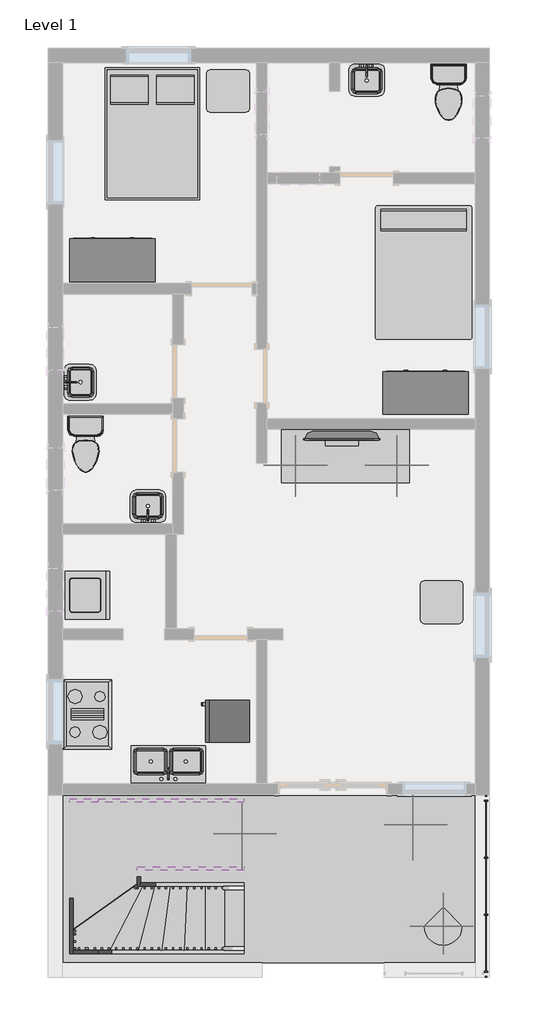
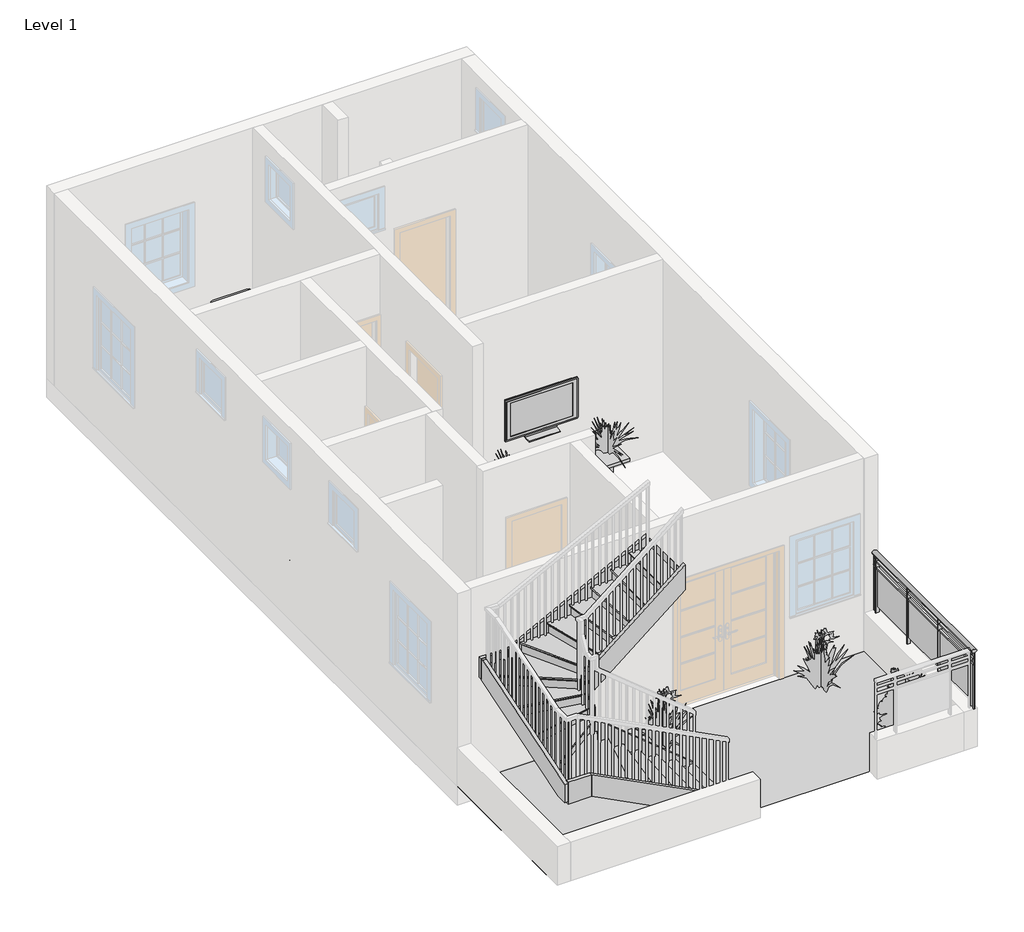
# One storey, part 3 of 3: 8 flow terminals, 8 furniture elements, 8 members, 5 geographic elements, 4 proxies, 1 railing, 1 stair flight.
"""IFC4 building model written with IfcOpenShell, lengths in millimetres."""

from ifc_helpers import new_model, si_unit, point, frame, origin, place, context, project, spatial, polyline, ellipse_curve, trimmed, outline, extrude, triangles, transform, mapped, element, save
from ifc_brep_helpers import plane_surface, extruded_surface, advanced_brep
from components import proxy_bb1e6e30, proxy_c523a7b7, proxy_718fa39f, flow_terminal_accce45a, flow_terminal_a53be723, flow_terminal_62a433f7, toilet_domestic_3d_toilet_domestic_3d_f7549cf7, toilet_domestic_3d_toilet_domestic_3d_183bbd19, furniture_c8abb964, furniture_0253826f, furniture_9fa109b2, furniture_7a3aaa4f, furniture_31d08a24, furniture_62ce4b1f, rpc_plant_tropical_55f6ff97, rpc_plant_tropical_agave_1_5_93a2a214, rpc_plant_tropical_jungle_flame_3_9c4808c2, stair_flight_52655b22

model = new_model("IFC4")

# Units and contexts
model_context = context("Model", 3, world=origin())
ifc_project = project(units=[si_unit("LENGTHUNIT", "METRE", prefix="MILLI")], contexts=[model_context])

# Site, building, storey
site = spatial("IfcSite", under=ifc_project)
building = spatial("IfcBuilding", under=site)
storey = spatial("IfcBuildingStorey", under=building, Name="Level 1", Elevation=0.0)

# Proxies
placement = place(None, origin())
element("IfcBuildingElementProxy", 1, Name="Building Element Proxy", at=placement, inside=storey, context=model_context, shape_type="Tessellation", body=[
    triangles([(-16060.3755066, 5665.9419479, 0.0), (-16060.3755066, 3354.5417542, 0.0), (-9761.1762817, 3354.5417542, 0.0), (-9761.1762817, 5665.9419479, 0.0), (-15857.1762817, 3278.3417542, 0.0), (-13012.3755066, 3278.3417542, 0.0), (-9964.3755066, 3278.3417542, 0.0)], [[1, 2, 5], [1, 5, 6], [6, 7, 4], [6, 4, 1], [3, 4, 7]], closed=False),
])
proxy_shape = proxy_bb1e6e30(model_context)
element("IfcBuildingElementProxy", 2, Name="Cook Top-4 Unit : 36\" x 20\"", ObjectType="Cook Top-4 Unit : 36\" x 20\"", at=placement, inside=storey, context=model_context, shape_type="MappedRepresentation", body=[
    mapped(proxy_shape, transform((-15501.5757671, 6821.6418963, 0.0), x_axis=(0.0, 1.0000000000000002, 0.0), y_axis=(-1.0000000000000002, 0.0, 0.0), z_axis=(0.0, 0.0, 1.0))),
])
proxy_2_shape = proxy_c523a7b7(model_context)
element("IfcBuildingElementProxy", 3, Name="Refrigerator : 24\" x 25\" LH", ObjectType="Refrigerator : 24\" x 25\" LH", at=placement, inside=storey, context=model_context, shape_type="MappedRepresentation", body=[
    mapped(proxy_2_shape, transform((-13488.6257671, 6725.1929248, 0.0), x_axis=(0.0, -1.0000000000000007, 0.0), y_axis=(1.0000000000000007, 0.0, 0.0), z_axis=(0.0, 0.0, 1.0))),
])
proxy_3_shape = proxy_718fa39f(model_context)
element("IfcBuildingElementProxy", 4, Name="Washer : 27\" x 25\" x 35\"", ObjectType="Washer : 27\" x 25\" x 35\"", at=placement, inside=storey, context=model_context, shape_type="MappedRepresentation", body=[
    mapped(proxy_3_shape, transform((-15782.2932356, 8942.7923315, 0.0), x_axis=(0.0, -1.0000000000000016, 0.0), y_axis=(1.0000000000000016, 0.0, 0.0), z_axis=(0.0, 0.0, 1.0))),
])

# Flow terminals
flow_terminal_shape = flow_terminal_accce45a(model_context)
element("IfcFlowTerminal", 5, ObjectType="Floor Drain - Round : 5\" Strainer - 2\" Drain", at=placement, inside=storey, context=model_context, shape_type="MappedRepresentation", body=[
    mapped(flow_terminal_shape, transform((-10294.5757671, 14873.4418963, 0.0), x_axis=(1.0, 0.0, 0.0), y_axis=(0.0, 1.0, 0.0), z_axis=(0.0, 0.0, 1.0))),
])
element("IfcFlowTerminal", 6, ObjectType="Floor Drain - Round : 5\" Strainer - 2\" Drain", at=placement, inside=storey, context=model_context, shape_type="MappedRepresentation", body=[
    mapped(flow_terminal_shape, transform((-15679.3757671, 12587.4418963, 0.0), x_axis=(1.0, 0.0, 0.0), y_axis=(0.0, 1.0, 0.0), z_axis=(0.0, 0.0, 1.0))),
])
flow_terminal_2_shape = flow_terminal_a53be723(model_context)
element("IfcFlowTerminal", 7, ObjectType="Sink Kitchen-Double : 42\" x 21\"", at=placement, inside=storey, context=model_context, shape_type="MappedRepresentation", body=[
    mapped(flow_terminal_2_shape, transform((-14330.1865265, 6112.7872974, 0.0), x_axis=(-1.0000000000000004, 0.0, 0.0), y_axis=(0.0, -1.0000000000000004, 0.0), z_axis=(0.0, 0.0, 1.0))),
])
flow_terminal_3_shape = flow_terminal_62a433f7(model_context)
element("IfcFlowTerminal", 8, ObjectType="Sink Vanity-Square : 20\" x 18\"", at=placement, inside=storey, context=model_context, shape_type="MappedRepresentation", body=[
    mapped(flow_terminal_3_shape, transform((-11529.4650076, 15912.4964952, 0.0), x_axis=(1.0, 0.0, 0.0), y_axis=(0.0, 1.0, 0.0), z_axis=(0.0, 0.0, 1.0))),
])
element("IfcFlowTerminal", 9, ObjectType="Sink Vanity-Square : 20\" x 18\"", at=placement, inside=storey, context=model_context, shape_type="MappedRepresentation", body=[
    mapped(flow_terminal_3_shape, transform((-15651.6303659, 11543.0526557, 0.0), x_axis=(0.0, 1.0, 0.0), y_axis=(-1.0, 0.0, 0.0), z_axis=(0.0, 0.0, 1.0))),
])
element("IfcFlowTerminal", 10, ObjectType="Sink Vanity-Square : 20\" x 18\"", at=placement, inside=storey, context=model_context, shape_type="MappedRepresentation", body=[
    mapped(flow_terminal_3_shape, transform((-14622.2865265, 9744.9872974, 0.0), x_axis=(-0.9999999999999998, 0.0, 0.0), y_axis=(0.0, -0.9999999999999998, 0.0), z_axis=(0.0, 0.0, 1.0))),
])
toilet_domestic_3d_toilet_domestic_3d_shape = toilet_domestic_3d_toilet_domestic_3d_f7549cf7(model_context)
toilet_domestic_3d_toilet_domestic_3d_2_shape = toilet_domestic_3d_toilet_domestic_3d_183bbd19(model_context)
element("IfcFlowTerminal", 11, ObjectType="Toilet-Domestic-3D : Toilet-Domestic-3D", at=placement, inside=storey, context=model_context, shape_type="MappedRepresentation", body=[
    mapped(toilet_domestic_3d_toilet_domestic_3d_shape, transform((-10345.3757671, 15597.9458689, 0.0), x_axis=(1.0, 0.0, 0.0), y_axis=(0.0, 1.0, 0.0), z_axis=(0.0, 0.0, 1.0))),
    mapped(toilet_domestic_3d_toilet_domestic_3d_2_shape, transform((-10345.3757671, 15597.9458689, 0.0), x_axis=(1.0, 0.0, 0.0), y_axis=(0.0, 1.0, 0.0), z_axis=(0.0, 0.0, 1.0))),
])
element("IfcFlowTerminal", 12, ObjectType="Toilet-Domestic-3D : Toilet-Domestic-3D", at=placement, inside=storey, context=model_context, shape_type="MappedRepresentation", body=[
    mapped(toilet_domestic_3d_toilet_domestic_3d_shape, transform((-15526.9757671, 10581.4458689, 0.0), x_axis=(1.0, 0.0, 0.0), y_axis=(0.0, 1.0, 0.0), z_axis=(0.0, 0.0, 1.0))),
    mapped(toilet_domestic_3d_toilet_domestic_3d_2_shape, transform((-15526.9757671, 10581.4458689, 0.0), x_axis=(1.0, 0.0, 0.0), y_axis=(0.0, 1.0, 0.0), z_axis=(0.0, 0.0, 1.0))),
])

# Furniture
furniture_shape = furniture_c8abb964(model_context)
element("IfcFurniture", 13, ObjectType="Bed-Box : Double 53\" x 74\"", at=placement, inside=storey, context=model_context, shape_type="MappedRepresentation", body=[
    mapped(furniture_shape, transform((-14913.6282261, 15336.4714045, 0.0), x_axis=(1.0, 0.0, 0.0), y_axis=(0.0, 1.0, 0.0), z_axis=(0.0, 0.0, 1.0))),
])
furniture_2_shape = furniture_0253826f(model_context)
element("IfcFurniture", 14, ObjectType="Bed-Standard.0001 : Double 54\" x 75\"", at=placement, inside=storey, context=model_context, shape_type="MappedRepresentation", body=[
    mapped(furniture_2_shape, transform((-10972.4642916, 13166.4369782, 0.0), x_axis=(1.0, 0.0, 0.0), y_axis=(0.0, 1.0, 0.0), z_axis=(0.0, 0.0, 1.0))),
])
furniture_3_shape = furniture_9fa109b2(model_context)
element("IfcFurniture", 15, ObjectType="Dresser : 48\" x 72\" x 24\"", at=placement, inside=storey, context=model_context, shape_type="MappedRepresentation", body=[
    mapped(furniture_3_shape, transform((-15415.1690269, 12935.4789422, 0.0), x_axis=(-1.0000000000000004, 0.0, 0.0), y_axis=(0.0, -1.0000000000000004, 0.0), z_axis=(0.0, 0.0, 1.0))),
])
element("IfcFurniture", 16, ObjectType="Dresser : 48\" x 72\" x 24\"", at=placement, inside=storey, context=model_context, shape_type="MappedRepresentation", body=[
    mapped(furniture_3_shape, transform((-10944.7690269, 11043.1789422, 0.0), x_axis=(-1.0000000000000004, 0.0, 0.0), y_axis=(0.0, -1.0000000000000004, 0.0), z_axis=(0.0, 0.0, 1.0))),
])
furniture_4_shape = furniture_7a3aaa4f(model_context)
element("IfcFurniture", 17, ObjectType="TV - Flat Screen : 42\"", at=placement, inside=storey, context=model_context, shape_type="MappedRepresentation", body=[
    mapped(furniture_4_shape, transform((-11865.4312529, 10801.7032726, 1041.4), x_axis=(1.0, 0.0, 0.0), y_axis=(0.0, 1.0, 0.0), z_axis=(0.0, 0.0, 1.0))),
])
furniture_5_shape = furniture_31d08a24(model_context)
element("IfcFurniture", 18, ObjectType="Table-End : 24\" x 24\"", at=placement, inside=storey, context=model_context, shape_type="MappedRepresentation", body=[
    mapped(furniture_5_shape, transform((-13803.5093973, 15559.2418963, 0.0), x_axis=(1.0, 0.0, 0.0), y_axis=(0.0, 1.0, 0.0), z_axis=(0.0, 0.0, 1.0))),
])
element("IfcFurniture", 19, ObjectType="Table-End : 24\" x 24\"", at=placement, inside=storey, context=model_context, shape_type="MappedRepresentation", body=[
    mapped(furniture_5_shape, transform((-10755.5093973, 8269.4418963, 0.0), x_axis=(1.0, 0.0, 0.0), y_axis=(0.0, 1.0, 0.0), z_axis=(0.0, 0.0, 1.0))),
])
furniture_6_shape = furniture_62ce4b1f(model_context)
element("IfcFurniture", 20, ObjectType="Table-Rectangular : 72\" x 30\"", at=placement, inside=storey, context=model_context, shape_type="MappedRepresentation", body=[
    mapped(furniture_6_shape, transform((-11818.5757671, 10504.6418963, 0.0), x_axis=(1.0, 0.0, 0.0), y_axis=(0.0, 1.0, 0.0), z_axis=(0.0, 0.0, 1.0))),
])

# Geographic elements
rpc_plant_tropical_shape = rpc_plant_tropical_55f6ff97(model_context)
element("IfcGeographicElement", 21, ObjectType="RPC Plant - Tropical", at=placement, inside=storey, context=model_context, shape_type="MappedRepresentation", body=[
    mapped(rpc_plant_tropical_shape, transform((-13291.7757671, 5119.8418963, 0.0), x_axis=(1.0, 0.0, 0.0), y_axis=(0.0, 1.0, 0.0), z_axis=(0.0, 0.0, 1.0))),
])
element("IfcGeographicElement", 22, ObjectType="RPC Plant - Tropical", at=placement, inside=storey, context=model_context, shape_type="MappedRepresentation", body=[
    mapped(rpc_plant_tropical_shape, transform((-10853.3757671, 5246.8418963, 0.0), x_axis=(1.0, 0.0, 0.0), y_axis=(0.0, 1.0, 0.0), z_axis=(0.0, 0.0, 1.0))),
])
rpc_plant_tropical_agave_1_5_shape = rpc_plant_tropical_agave_1_5_93a2a214(model_context)
element("IfcGeographicElement", 23, ObjectType="RPC Plant - Tropical : Agave - 1.5'", at=placement, inside=storey, context=model_context, shape_type="MappedRepresentation", body=[
    mapped(rpc_plant_tropical_agave_1_5_shape, transform((-12529.7757671, 10377.6418963, 685.8), x_axis=(1.0, 0.0, 0.0), y_axis=(0.0, 1.0, 0.0), z_axis=(0.0, 0.0, 1.0))),
])
element("IfcGeographicElement", 24, ObjectType="RPC Plant - Tropical : Agave - 1.5'", at=placement, inside=storey, context=model_context, shape_type="MappedRepresentation", body=[
    mapped(rpc_plant_tropical_agave_1_5_shape, transform((-11081.9757671, 10377.6418963, 685.8), x_axis=(1.0, 0.0, 0.0), y_axis=(0.0, 1.0, 0.0), z_axis=(0.0, 0.0, 1.0))),
])
rpc_plant_tropical_jungle_flame_3_shape = rpc_plant_tropical_jungle_flame_3_9c4808c2(model_context)
element("IfcGeographicElement", 25, ObjectType="RPC Plant - Tropical : Jungle Flame - 3'", at=placement, inside=storey, context=model_context, shape_type="MappedRepresentation", body=[
    mapped(rpc_plant_tropical_jungle_flame_3_shape, transform((-10421.5757671, 3799.0418963, 0.0), x_axis=(1.0, 0.0, 0.0), y_axis=(0.0, 1.0, 0.0), z_axis=(0.0, 0.0, 1.0))),
])

# Members
element("IfcMember", 26, ObjectType="Stringer - 2\" Width", at=placement, inside=storey, context=model_context, shape_type="SweptSolid", body=[
    extrude(outline(polyline([(0.0, -13262.6440752), (229.639954, -13262.6440752), (1305.3956453, -15350.0612669), (962.500629, -15350.0612669), (0.0, -13482.4063928), (0.0, -13262.6440752)])), frame((0.0, 3405.3418963, 0.0), z_axis=(0.0, 1.0, 0.0), x_axis=(0.0, 0.0, 1.0)), (0.0, 0.0, 1.0), 50.8),
])
element("IfcMember", 27, ObjectType="Stringer - 2\" Width", at=placement, inside=storey, context=model_context, shape_type="SweptSolid", body=[
    extrude(outline(polyline([(-15350.0612669, 3456.1418963), (-15350.0612669, 3405.3418963), (-15704.7757671, 3405.3418963), (-15704.7757671, 3456.1418963), (-15350.0612669, 3456.1418963)])), frame((0.0, 0.0, 962.500629), z_axis=(0.0, 0.0, 1.0), x_axis=(1.0, 0.0, 0.0)), (0.0, 0.0, 1.0), 342.8950162),
])
element("IfcMember", 28, ObjectType="Stringer - 2\" Width", at=placement, inside=storey, context=model_context, shape_type="SweptSolid", body=[
    extrude(outline(polyline([(3405.3418963, 1000.5956453), (3405.3418963, 1289.0952212), (5527.361779, 1969.9972697), (5564.3418963, 1969.9972697), (5564.3418963, 1638.9682298), (3574.8643792, 1000.5956453), (3405.3418963, 1000.5956453)])), frame((-15755.5757671, 0.0, 0.0), z_axis=(1.0, 0.0, 0.0), x_axis=(0.0, 1.0, 0.0)), (0.0, 0.0, 1.0), 50.8),
])
element("IfcMember", 29, ObjectType="Stringer - 2\" Width", at=placement, inside=storey, context=model_context, shape_type="SweptSolid", body=[
    extrude(outline(polyline([(-15755.5757671, 5564.3418963), (-15755.5757671, 5615.1418963), (-15350.0612669, 5615.1418963), (-15350.0612669, 5564.3418963), (-15755.5757671, 5564.3418963)])), frame((0.0, 0.0, 1649.8904473), z_axis=(0.0, 0.0, 1.0), x_axis=(1.0, 0.0, 0.0)), (0.0, 0.0, 1.0), 320.1068224),
])
element("IfcMember", 30, ObjectType="Stringer - 2\" Width", at=placement, inside=storey, context=model_context, shape_type="SweptSolid", body=[
    extrude(outline(polyline([(1969.9972697, -15350.0612669), (1649.8904473, -15350.0612669), (2725.6461385, -13262.6440752), (3045.7529609, -13262.6440752), (1969.9972697, -15350.0612669)])), frame((0.0, 5564.3418963, 0.0), z_axis=(0.0, 1.0, 0.0), x_axis=(0.0, 0.0, 1.0)), (0.0, 0.0, 1.0), 50.8),
])
element("IfcMember", 31, ObjectType="Stringer - 2\" Width", at=placement, inside=storey, context=model_context, shape_type="SweptSolid", body=[
    extrude(outline(polyline([(0.0, -13262.6440752), (176.1764461, -13262.6440752), (1380.418648, -14739.5757671), (987.1410923, -14739.5757671), (0.0, -13528.9057197), (0.0, -13262.6440752)])), frame((0.0, 4370.5418963, 0.0), z_axis=(0.0, 1.0, 0.0), x_axis=(0.0, 0.0, 1.0)), (0.0, 0.0, 1.0), 50.8),
])
element("IfcMember", 32, ObjectType="Stringer - 2\" Width", at=placement, inside=storey, context=model_context, shape_type="SweptSolid", body=[
    extrude(outline(polyline([(4370.5418963, 1028.5617647), (4370.5418963, 1573.2682978), (4577.1790137, 1926.1409689), (4599.1418963, 1926.1409689), (4599.1418963, 1360.465107), (4404.7841136, 1028.5617647), (4370.5418963, 1028.5617647)])), frame((-14790.3757671, 0.0, 0.0), z_axis=(1.0, 0.0, 0.0), x_axis=(0.0, 1.0, 0.0)), (0.0, 0.0, 1.0), 50.8),
])
element("IfcMember", 33, ObjectType="Stringer - 2\" Width", at=placement, inside=storey, context=model_context, shape_type="SweptSolid", body=[
    extrude(outline(polyline([(1926.1409689, -14790.3757671), (1532.8634131, -14790.3757671), (2778.5262875, -13262.6440752), (3171.8038432, -13262.6440752), (1926.1409689, -14790.3757671)])), frame((0.0, 4599.1418963, 0.0), z_axis=(0.0, 1.0, 0.0), x_axis=(0.0, 0.0, 1.0)), (0.0, 0.0, 1.0), 50.8),
])

# Railing
element("IfcRailing", 34, ObjectType="Glass Panel - Bottom Fill", at=placement, inside=storey, context=model_context, shape_type="SolidModel", body=[
    advanced_brep(
    [(-9773.8757671, 5665.9418963, 1524.0), (-9850.0757671, 5665.9418963, 1524.0), (-9773.8757671, 3075.1418963, 1524.0), (-9850.0757671, 3075.1418963, 1524.0)],
    [
        (0, 1, ellipse_curve(frame((-9811.9757671, 5665.9418963, 1524.0), z_axis=(0.0, 1.0, 0.0), x_axis=(-1.0, 0.0, 0.0)), 38.1, 28.575)),
        (1, 0, ellipse_curve(frame((-9811.9757671, 5665.9418963, 1524.0), z_axis=(0.0, 1.0, 0.0), x_axis=(-1.0, 0.0, 0.0)), 38.1, 28.575)),
        (2, 3, ellipse_curve(frame((-9811.9757671, 3075.1418963, 1524.0), z_axis=(0.0, -1.0, 0.0), x_axis=(-1.0, 0.0, 0.0)), 38.1, 28.575)),
        (3, 2, ellipse_curve(frame((-9811.9757671, 3075.1418963, 1524.0), z_axis=(0.0, -1.0, 0.0), x_axis=(-1.0, 0.0, 0.0)), 38.1, 28.575)),
        (0, 2),
        (3, 1),
    ],
    [
        plane_surface(frame((-9811.9757671, 5665.9418963, 1524.0), z_axis=(0.0, 1.0, 0.0), x_axis=(0.0, 0.0, -1.0))),
        plane_surface(frame((-9811.9757671, 3075.1418963, 1524.0), z_axis=(0.0, -1.0, 0.0), x_axis=(0.0, 0.0, -1.0))),
        extruded_surface(trimmed(ellipse_curve(frame((-9811.9757671, 3075.1418963, 1524.0), z_axis=(0.0, 1.0, 0.0), x_axis=(-1.0, 0.0, 0.0)), 38.1, 28.575), [point((-9773.8757671, 3075.1418963, 1524.0))], [point((-9850.0757671, 3075.1418963, 1524.0))], True, "CARTESIAN"), (0.0, 2590.7999999999997, 0.0), 2590.7999999999997),
        extruded_surface(trimmed(ellipse_curve(frame((-9811.9757671, 3075.1418963, 1524.0), z_axis=(0.0, 1.0, 0.0), x_axis=(-1.0, 0.0, 0.0)), 38.1, 28.575), [point((-9850.0757671, 3075.1418963, 1524.0))], [point((-9773.8757671, 3075.1418963, 1524.0))], True, "CARTESIAN"), (0.0, 2590.7999999999997, 0.0), 2590.7999999999997),
    ],
    [
        (0, [[1, 2]]),
        (1, [[3, 4]]),
        (2, [[-1, 5, -4, 6]]),
        (3, [[-2, -6, -3, -5]]),
    ],
),
    extrude(outline(polyline([(-9824.6757671, 5665.9418963), (-9799.2757671, 5665.9418963), (-9799.2757671, 3075.1418963), (-9824.6757671, 3075.1418963), (-9824.6757671, 5665.9418963)])), frame((0.0, 0.0, 1409.7), z_axis=(0.0, 0.0, 1.0), x_axis=(1.0, 0.0, 0.0)), (0.0, 0.0, 1.0), 25.4),
    extrude(outline(polyline([(-9824.6757671, 5665.9418963), (-9799.2757671, 5665.9418963), (-9799.2757671, 3075.1418963), (-9824.6757671, 3075.1418963), (-9824.6757671, 5665.9418963)])), frame((0.0, 0.0, 1308.1), z_axis=(0.0, 0.0, 1.0), x_axis=(1.0, 0.0, 0.0)), (0.0, 0.0, 1.0), 25.4),
    extrude(outline(polyline([(-9837.3757671, 3157.6918963), (-9786.5757671, 3157.6918963), (-9786.5757671, 3144.9918963), (-9837.3757671, 3144.9918963), (-9837.3757671, 3157.6918963)])), frame((0.0, 0.0, 609.6), z_axis=(0.0, 0.0, 1.0), x_axis=(1.0, 0.0, 0.0)), (0.0, 0.0, 1.0), 885.6788223),
    extrude(outline(polyline([(-9805.4406101, 3964.1418963), (-9805.4406101, 3151.3418963), (-9811.7906101, 3151.3418963), (-9811.7906101, 3964.1418963), (-9805.4406101, 3964.1418963)])), frame((0.0, 0.0, 711.2), z_axis=(0.0, 0.0, 1.0), x_axis=(1.0, 0.0, 0.0)), (0.0, 0.0, 1.0), 596.9),
    extrude(outline(polyline([(-9837.3757671, 3970.4918963), (-9786.5757671, 3970.4918963), (-9786.5757671, 3957.7918963), (-9837.3757671, 3957.7918963), (-9837.3757671, 3970.4918963)])), frame((0.0, 0.0, 609.6), z_axis=(0.0, 0.0, 1.0), x_axis=(1.0, 0.0, 0.0)), (0.0, 0.0, 1.0), 885.6788223),
    extrude(outline(polyline([(-9805.4406101, 4776.9418963), (-9805.4406101, 3964.1418963), (-9811.7906101, 3964.1418963), (-9811.7906101, 4776.9418963), (-9805.4406101, 4776.9418963)])), frame((0.0, 0.0, 711.2), z_axis=(0.0, 0.0, 1.0), x_axis=(1.0, 0.0, 0.0)), (0.0, 0.0, 1.0), 596.9),
    extrude(outline(polyline([(-9837.3757671, 4783.2918963), (-9786.5757671, 4783.2918963), (-9786.5757671, 4770.5918963), (-9837.3757671, 4770.5918963), (-9837.3757671, 4783.2918963)])), frame((0.0, 0.0, 609.6), z_axis=(0.0, 0.0, 1.0), x_axis=(1.0, 0.0, 0.0)), (0.0, 0.0, 1.0), 885.6788223),
    extrude(outline(polyline([(-9805.4406101, 5589.7418963), (-9805.4406101, 4776.9418963), (-9811.7906101, 4776.9418963), (-9811.7906101, 5589.7418963), (-9805.4406101, 5589.7418963)])), frame((0.0, 0.0, 711.2), z_axis=(0.0, 0.0, 1.0), x_axis=(1.0, 0.0, 0.0)), (0.0, 0.0, 1.0), 596.9),
    extrude(outline(polyline([(-9837.3757671, 5596.0918963), (-9786.5757671, 5596.0918963), (-9786.5757671, 5583.3918963), (-9837.3757671, 5583.3918963), (-9837.3757671, 5596.0918963)])), frame((0.0, 0.0, 609.6), z_axis=(0.0, 0.0, 1.0), x_axis=(1.0, 0.0, 0.0)), (0.0, 0.0, 1.0), 885.6788223),
    extrude(outline(polyline([(-9821.5007671, 3087.8418963), (-9802.4507671, 3087.8418963), (-9802.4507671, 3068.7918963), (-9821.5007671, 3068.7918963), (-9821.5007671, 3087.8418963)])), frame((0.0, 0.0, 609.6), z_axis=(0.0, 0.0, 1.0), x_axis=(1.0, 0.0, 0.0)), (0.0, 0.0, 1.0), 885.6788223),
    extrude(outline(polyline([(-9821.5007671, 5672.2918963), (-9802.4507671, 5672.2918963), (-9802.4507671, 5653.2418963), (-9821.5007671, 5653.2418963), (-9821.5007671, 5672.2918963)])), frame((0.0, 0.0, 609.6), z_axis=(0.0, 0.0, 1.0), x_axis=(1.0, 0.0, 0.0)), (0.0, 0.0, 1.0), 885.6788223),
])

# Stair flight
stair_flight_shape = stair_flight_52655b22(model_context)
element("IfcStairFlight", 35, ObjectType="2\" Tread 1\" Nosing 1/4\" Riser", at=placement, inside=storey, context=model_context, shape_type="MappedRepresentation", body=[
    mapped(stair_flight_shape, transform((0.0, 0.0, 0.0), x_axis=(1.0, 0.0, 0.0), y_axis=(0.0, 1.0, 0.0), z_axis=(0.0, 0.0, 1.0))),
])

save(model, "model.ifc")

# Revit data of these elements
# Type "Cook Top-4 Unit : 36\" x 20\""
#   Assembly Code = "E1090400"
#   Depth = 2' - 0"
#   Width = 3' - 0"
#   Burner Material = Steel, Chrome Plated
#   Cooktop Material = Steel, Polished
#   Default Elevation = 0
# Type "Refrigerator : 24\" x 25\" LH"
#   Label = "REF."
#   Assembly Code = "E1090400"
#   Depth = 2' - 0 3/4"
#   Handle = 0' - 1 1/2"
#   Height = 5' - 3 1/2"
#   Rear Clearance = 0' - 2"
#   Top Door Height = 1' - 8"
#   Width = 1' - 11 1/2"
#   Material = Steel, Paint Finish, Ivory, Glossy
#   Default Elevation = 0
# Type "Washer : 27\" x 25\" x 35\""
#   Label = "W"
#   Assembly Code = "E1090400"
#   Depth = 2' - 1"
#   Height = 2' - 11"
#   Width = 2' - 3"
#   Washer Material = Steel, Paint Finish, Ivory, Matte
#   Default Elevation = 0
# Type "Floor Drain - Round : 5\" Strainer - 2\" Drain"
#   WFU = 2
#   Strainer Height = 0' - 3 1/4"
#   Strainer Radius = 0' - 2 1/2"
#   Strainer Diameter = 0' - 5"
#   Radius 6 = 0' - 0 5/8"
#   Radius 5 = 0' - 1 1/4"
#   Radius 4 = 0' - 1 7/8"
#   Radius 2 = 0' - 3.04167"
#   Radius 1 = 0' - 2.02083"
#   Radius 3 = 0' - 2 1/32"
#   Pipe Radius = 1"
#   Pipe Diameter = 2"
#   Height 2 = 0' - 0.725"
#   Height 1 = 0' - 1 13/16"
#   Body Radius = 0' - 4 1/16"
#   Body Height = 0' - 3 5/8"
#   Body Diameter = 0' - 8 1/8"
#   Drain Material = none
#   HWFU = 0
#   Default Elevation = 0
#   CWFU = 0
# Type "Sink Kitchen-Double : 42\" x 21\""
#   Assembly Code = "D2010410"
#   Counter Height = 3' - 0"
#   Depth = 1' - 9"
#   Width = 3' - 6"
#   Faucet Material = Steel, Polished
#   Sink Material = Steel, Polished
#   Default Elevation = 0
# Type "Sink Vanity-Square : 20\" x 18\""
#   Assembly Code = "D2010400"
#   Counter Height = 2' - 7"
#   Depth = 1' - 6"
#   Width = 1' - 8"
#   Basin Material = Porcelain, Linen
#   Faucet Material = Steel, Polished
#   Default Elevation = 0
# Type "Toilet-Domestic-3D : Toilet-Domestic-3D"
#   Assembly Code = "D2010110"
#   Toilet - Bowl/Basin Material = Porcelain, Linen
#   Toilet - Seat Material = Laminate, Linen, Matte
#   Default Elevation = 0
# Type "Bed-Box : Double 53\" x 74\""
#   Assembly Code = "E2020200"
#   Length = 6' - 2"
#   Width = 4' - 5"
#   Frame Material = Birch
#   Mattress Material = Linen, White
#   Default Elevation = 0
# Type "Bed-Standard.0001 : Double 54\" x 75\""
#   Assembly Code = "E2020200"
#   Length = 6' - 3"
#   Width = 4' - 6"
#   Leg Material = Steel, Chrome Plated
#   Mattress Material = Linen, White
#   Default Elevation = 0
# Type "Dresser : 48\" x 72\" x 24\""
#   Assembly Code = "E2020200"
#   Depth = 2' - 0"
#   Height = 6' - 0"
#   Width = 4' - 0"
#   Dresser Material = Laminate - Ivory, Glossy
#   Drawer Material = Laminate, Ivory, Matte
#   Knob Material = Cherry
#   Default Elevation = 0
# Type "TV - Flat Screen : 42\""
#   SinAng = 0' - 0.0193"
#   L = 3' - 0.71517"
#   H = 1' - 8.65418"
#   Thickness = 0' - 4.33071"
#   Diagonal = 3' - 6.12598"
#   CosAng = 0' - 0.03431"
#   Stand [instance default] = yes
#   Default Elevation = 0
# Type "Table-End : 24\" x 24\""
#   Assembly Code = "E2020200"
#   Height = 2' - 0"
#   Length = 2' - 0"
#   Width = 2' - 0"
#   Base Material = Birch
#   Top Material = Laminate, Ivory, Matte
#   Default Elevation = 0
# Type "Table-Rectangular : 72\" x 30\""
#   Assembly Code = "E2020200"
#   Height = 2' - 3"
#   Length = 6' - 0"
#   Width = 2' - 6"
#   Base Material = Birch
#   Top Material = Birch
#   Default Elevation = 0
# Type "RPC Plant - Tropical"
#   built-in parameter 1005198 = "{2, 15},{39, RPC-16-FWM5-GM7X-C67P-4000-ST1L-LVER-AU},{1, 0},{1, 0},{2, 13},{1, 8},{5, Color},{1, 0},{1, 0},{3, 0.8},{3, 0.8},{3, 0.8},{1, 8},{7, BBoxMin},{1, 0},{1, 0},{1, 0},{1, 0},{1, 0},{1, 8},{7, BBoxMax},{1, 0},{1, 0},{1, 0},{1, 0},{1, 0},{2, 11},{9, RPCTypeId},{1, 0},{1, 0},{39, RPC-16-FWM5-GM7X-C67P-4000-ST1L-LVER-AU},{1, 6},{14, RPCPlantHeight},{1, 0},{1, 0},{1, 3},{2, 11},{7, keyword},{1, 0},{1, 0},{35, :RPCs:Shrubs [General]:Geometry:RPC},{2, 11},{8, category},{1, 0},{1, 0},{16, Shrubs [General]},{2, 11},{12, LocalizedUID},{1, 0},{1, 0},{10, Crane Lily},{2, 14},{6, Height},{1, 0},{1, 0},{1, 3},{1, 2},{16, Cast Reflections},{1, 0},{1, 0},{1, 0},{1, 2},{12, Cast Shadows},{1, 0},{1, 0},{1, 1},{1, 2},{9, Lock View},{1, 0},{1, 0},{1, 0},{1, 4},{5, ViewC},{1, 0},{1, 0},{1, 0},{21, assetlibrary_base.fbx},{1, 5},"
#   built-in parameter 1005195 = "RPC-16-FWM5-GM7X-C67P-4000-ST1L-LVER-AU"
#   Assembly Code = "G2050500"
#   Height = 3' - 0"
#   Default Elevation = 0
# Type "RPC Plant - Tropical : Agave - 1.5'"
#   built-in parameter 1005198 = "{2, 15},{39, RPC-16-G1GJ-63FX-7K5P-N000-ST1L-LVER-AU},{1, 0},{1, 0},{2, 13},{1, 8},{5, Color},{1, 0},{1, 0},{3, 0.8},{3, 0.8},{3, 0.8},{1, 8},{7, BBoxMin},{1, 0},{1, 0},{1, 0},{1, 0},{1, 0},{1, 8},{7, BBoxMax},{1, 0},{1, 0},{1, 0},{1, 0},{1, 0},{2, 11},{9, RPCTypeId},{1, 0},{1, 0},{39, RPC-16-G1GJ-63FX-7K5P-N000-ST1L-LVER-AU},{1, 6},{14, RPCPlantHeight},{1, 0},{1, 0},{3, 1.5},{2, 11},{7, keyword},{1, 0},{1, 0},{35, :RPCs:Plants [General]:Geometry:RPC},{2, 11},{8, category},{1, 0},{1, 0},{16, Plants [General]},{2, 11},{12, LocalizedUID},{1, 0},{1, 0},{5, Agave},{2, 14},{6, Height},{1, 0},{1, 0},{3, 1.5},{1, 2},{16, Cast Reflections},{1, 0},{1, 0},{1, 0},{1, 2},{12, Cast Shadows},{1, 0},{1, 0},{1, 1},{1, 2},{9, Lock View},{1, 0},{1, 0},{1, 0},{1, 4},{5, ViewC},{1, 0},{1, 0},{1, 0},{21, assetlibrary_base.fbx},{1, 5},"
#   built-in parameter 1005195 = "RPC-16-G1GJ-63FX-7K5P-N000-ST1L-LVER-AU"
#   Type Comments = "Agave"
#   Assembly Code = "G2050500"
#   Height = 1' - 6"
#   Default Elevation = 0
# Type "RPC Plant - Tropical : Jungle Flame - 3'"
#   built-in parameter 1005198 = "{2, 15},{39, RPC-16-FUVJ-JWG0-MWGK-8000-ST1L-LVER-AU},{1, 0},{1, 0},{2, 13},{1, 8},{5, Color},{1, 0},{1, 0},{3, 0.8},{3, 0.8},{3, 0.8},{1, 8},{7, BBoxMin},{1, 0},{1, 0},{1, 0},{1, 0},{1, 0},{1, 8},{7, BBoxMax},{1, 0},{1, 0},{1, 0},{1, 0},{1, 0},{2, 11},{9, RPCTypeId},{1, 0},{1, 0},{39, RPC-16-FUVJ-JWG0-MWGK-8000-ST1L-LVER-AU},{1, 6},{14, RPCPlantHeight},{1, 0},{1, 0},{1, 3},{2, 11},{7, keyword},{1, 0},{1, 0},{35, :RPCs:Shrubs [General]:Geometry:RPC},{2, 11},{8, category},{1, 0},{1, 0},{16, Shrubs [General]},{2, 11},{12, LocalizedUID},{1, 0},{1, 0},{12, Jungle Flame},{2, 14},{6, Height},{1, 0},{1, 0},{1, 3},{1, 2},{16, Cast Reflections},{1, 0},{1, 0},{1, 0},{1, 2},{12, Cast Shadows},{1, 0},{1, 0},{1, 1},{1, 2},{9, Lock View},{1, 0},{1, 0},{1, 0},{1, 4},{5, ViewC},{1, 0},{1, 0},{1, 0},{21, assetlibrary_base.fbx},{1, 5},"
#   built-in parameter 1005195 = "RPC-16-FUVJ-JWG0-MWGK-8000-ST1L-LVER-AU"
#   Type Comments = "Jungle Flame"
#   Assembly Code = "G2050500"
#   Height = 3' - 0"
#   Default Elevation = 0
# Type "Glass Panel - Bottom Fill"
#   Assembly Code = "C2010400"
#   built-in parameter 1008612 = 0.0416667 (stored number, unit not read)
#   built-in parameter 1008611 = 0.0416667 (stored number, unit not read)
#   built-in parameter 1008609 = 0.333333 (stored number, unit not read)
#   built-in parameter 1008604 = 0.166667 (stored number, unit not read)
#   built-in parameter 1008603 = 0.166667 (stored number, unit not read)
#   Railing Height = 3' - 0"
#   built-in parameter 1008630 = 2
#   built-in parameter 1008610 = 2
#   built-in parameter 1008618 = Baluster - Square : 3/4"
# Element 1 (IfcBuildingElementProxy)
#   Material = none
#   Phase Created = New Construction
# Element 2 (IfcBuildingElementProxy, "Cook Top-4 Unit : 36\" x 20\"")
#   Phase Created = New Construction
#   Materials on its faces: "Steel, Chrome Plated", "Steel, Polished"
# Element 3 (IfcBuildingElementProxy, "Refrigerator : 24\" x 25\" LH")
#   Phase Created = New Construction
#   Materials on its faces: "Steel, Paint Finish, Ivory, Glossy", "Steel, Chrome Plated"
# Element 4 (IfcBuildingElementProxy, "Washer : 27\" x 25\" x 35\"")
#   Phase Created = New Construction
#   Materials on its faces: "Steel, Paint Finish, Ivory, Matte"
# Element 5 (IfcFlowTerminal, "Floor Drain - Round : 5\" Strainer - 2\" Drain")
#   Mark = "3"
#   Phase Created = New Construction
# Element 6 (IfcFlowTerminal, "Floor Drain - Round : 5\" Strainer - 2\" Drain")
#   Mark = "6"
#   Phase Created = New Construction
# Element 7 (IfcFlowTerminal, "Sink Kitchen-Double : 42\" x 21\"")
#   Mark = "9"
#   Phase Created = New Construction
#   Materials on its faces: "Steel, Polished"
# Element 8 (IfcFlowTerminal, "Sink Vanity-Square : 20\" x 18\"")
#   Mark = "2"
#   Phase Created = New Construction
#   Materials on its faces: "Porcelain, Linen", "Steel, Polished"
# Element 9 (IfcFlowTerminal, "Sink Vanity-Square : 20\" x 18\"")
#   Mark = "5"
#   Phase Created = New Construction
#   Materials on its faces: "Porcelain, Linen", "Steel, Polished"
# Element 10 (IfcFlowTerminal, "Sink Vanity-Square : 20\" x 18\"")
#   Mark = "8"
#   Phase Created = New Construction
#   Materials on its faces: "Porcelain, Linen", "Steel, Polished"
# Element 11 (IfcFlowTerminal, "Toilet-Domestic-3D : Toilet-Domestic-3D")
#   Mark = "1"
#   Phase Created = New Construction
#   Materials on its faces: "Porcelain, Linen", "Laminate, Linen, Matte"
# Element 12 (IfcFlowTerminal, "Toilet-Domestic-3D : Toilet-Domestic-3D")
#   Mark = "7"
#   Phase Created = New Construction
#   Materials on its faces: "Porcelain, Linen", "Laminate, Linen, Matte"
# Element 13 (IfcFurniture, "Bed-Box : Double 53\" x 74\"")
#   Phase Created = New Construction
#   Materials on its faces: "Birch", "Linen, White"
# Element 14 (IfcFurniture, "Bed-Standard.0001 : Double 54\" x 75\"")
#   Phase Created = New Construction
#   Materials on its faces: "Linen, White", "Steel, Chrome Plated"
# Elements 15, 16 (IfcFurniture, "Dresser : 48\" x 72\" x 24\"")
#   Phase Created = New Construction
#   Materials on its faces: "Laminate, Ivory, Matte", "Cherry", "Laminate - Ivory, Glossy"
# Element 17 (IfcFurniture, "TV - Flat Screen : 42\"")
#   Stand = yes
#   Phase Created = New Construction
#   Materials on its faces: "TV - Black", "TV - Glass", "TV - Screen"
# Elements 18, 19 (IfcFurniture, "Table-End : 24\" x 24\"")
#   Phase Created = New Construction
#   Materials on its faces: "Laminate, Ivory, Matte", "Birch"
# Element 20 (IfcFurniture, "Table-Rectangular : 72\" x 30\"")
#   Phase Created = New Construction
#   Materials on its faces: "Birch"
# Elements 21, 22 (IfcGeographicElement, "RPC Plant - Tropical")
#   Phase Created = New Construction
# Elements 23, 24 (IfcGeographicElement, "RPC Plant - Tropical : Agave - 1.5'")
#   Phase Created = New Construction
# Element 25 (IfcGeographicElement, "RPC Plant - Tropical : Jungle Flame - 3'")
#   Phase Created = New Construction
# Elements 26, 27, 28, 29, 30, 31, 32, 33 (IfcMember, "Stringer - 2\" Width")
#   Phase Created = New Construction
# Element 34 (IfcRailing, "Glass Panel - Bottom Fill")
#   built-in parameter 1008621 = 2 (stored number, unit not read)
#   Phase Created = New Construction
#   Materials on its faces: "Glass"
# Element 35 (IfcStairFlight, "2\" Tread 1\" Nosing 1/4\" Riser")
#   Phase Created = New Construction
# Materials
#   "Steel, Chrome Plated": class "Metal", colour RGB 17 17 17, transparency 0, Description = "Chromiuim plated steel", Cost = 0
#   "Steel, Polished": class "Metal", colour RGB 57 57 57, transparency 0, Description = "Polished steel", Cost = 0
#   "Steel, Paint Finish, Ivory, Glossy": class "Metal", colour RGB 247 247 239, transparency 0, Description = "Steel, paint finish, ivory, glossy", Cost = 0
#   "Steel, Paint Finish, Ivory, Matte": class "Metal", colour RGB 247 247 239, transparency 0, Description = "Steel, paint finish, ivory, matte", Cost = 0
#   "Porcelain, Linen": class "Ceramic", colour RGB 249 239 230, transparency 0, Description = "Porcelain, linen", Cost = 0
#   "Laminate, Linen, Matte": class "Plastic", colour RGB 249 239 230, transparency 0, Description = "Plastic Laminate - Linen, Matte", Cost = 0
#   "Birch": class "Wood", colour RGB 224 178 126, transparency 0, Description = "Betula Alleghaniensis", Cost = 0
#   "Linen, White": class "Textile", colour RGB 247 247 239, transparency 0, Description = "Linen, white", Cost = 0
#   "Laminate - Ivory, Glossy": colour RGB 247 247 239, transparency 0
#   "Laminate, Ivory, Matte": class "Plastic", colour RGB 247 247 239, transparency 0, Description = "Plastic Laminate - Ivory, Matte", Cost = 0
#   "Cherry": class "Wood", colour RGB 226 177 128, transparency 0, Description = "Prunus Serotina", Cost = 0
#   "TV - Black": colour RGB 49 49 49, transparency 0
#   "TV - Glass": colour RGB 157 157 157, transparency 0.9
#   "TV - Screen": colour RGB 0 0 0, transparency 0
#   "Glass": class "Glass", colour RGB 0 128 192, transparency 0.75, Description = "Soda Lime Glass", Cost = 0
